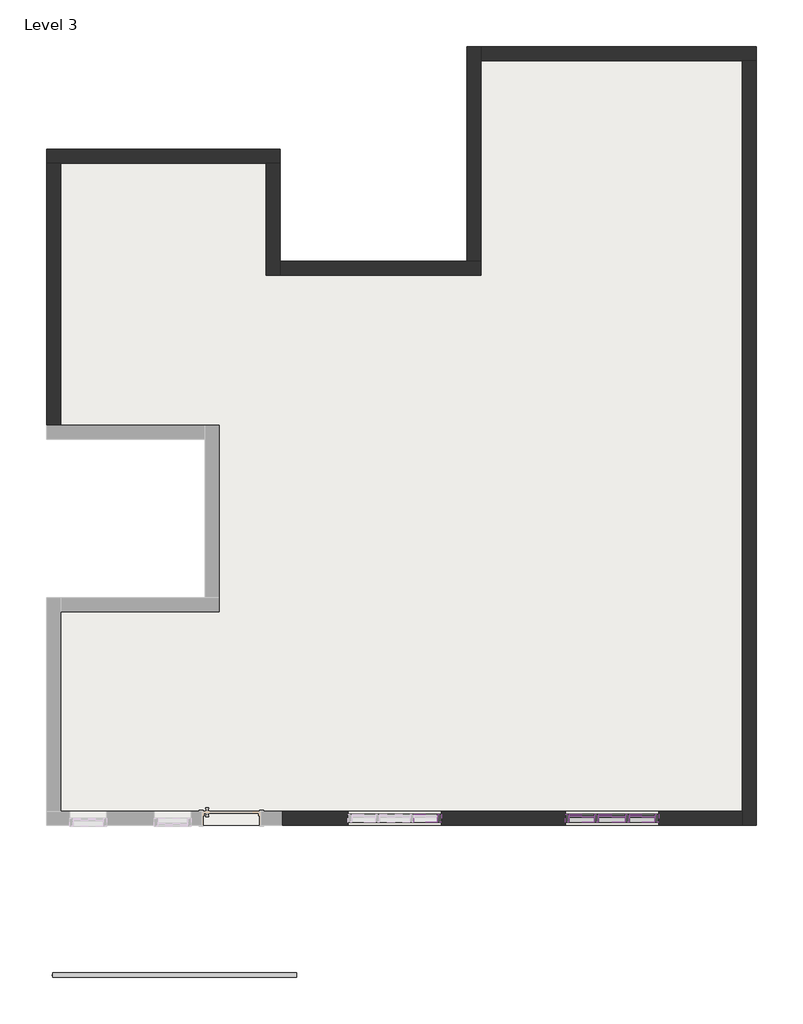
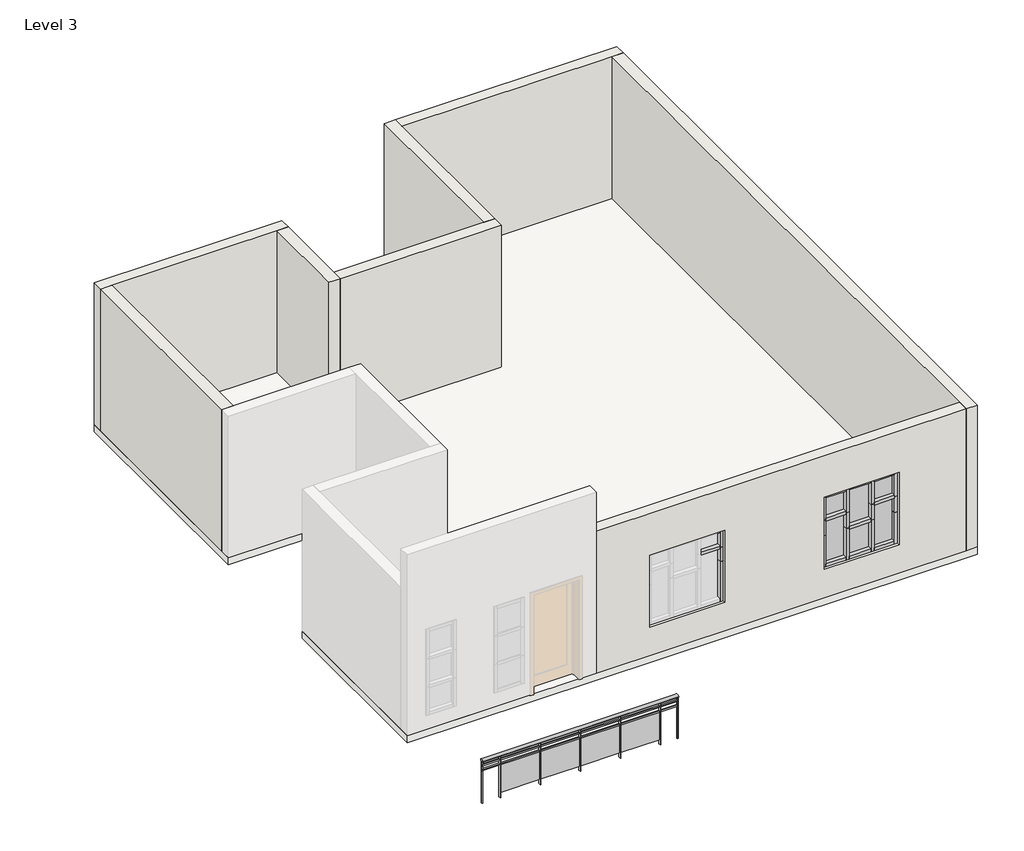
# One storey, part 2 of 2: 25 members, 8 walls, 6 plates, 1 railing, 1 slab.
"""IFC4 building model written with IfcOpenShell, lengths in millimetres."""

from ifc_helpers import new_model, si_unit, point, frame, origin, place, context, project, spatial, polyline, ellipse_curve, trimmed, outline, extrude, faceted_brep, transform, mapped, element, save
from ifc_brep_helpers import plane_surface, extruded_surface, advanced_brep
from components import member_3709dd30, member_b70ee1cc, member_3c3dc66a, member_dfe75557, member_dc106669, member_6428e230, member_5ae8a700, member_718fe5d9, member_bc7dbe04, member_b2812fca, member_26d576e8, member_fb4dac25, member_bdfbb35d, member_b281fab0, system_panel_glazed_1c8147a1, system_panel_glazed_d072c6ac, system_panel_glazed_ee3fb3da, system_panel_glazed_af2b4658

model = new_model("IFC4")

# Units and contexts
model_context = context("Model", 3, world=origin())
ifc_project = project(units=[si_unit("LENGTHUNIT", "METRE", prefix="MILLI")], contexts=[model_context])

# Site, building, storey
site = spatial("IfcSite", under=ifc_project)
building = spatial("IfcBuilding", under=site)
storey = spatial("IfcBuildingStorey", under=building, Name="Level 3", Elevation=3810.0)

# Members
placement = place(None, origin())
member_shape = member_3709dd30(model_context)
element("IfcMember", 1, ObjectType="Rectangular Mullion : 2.5\" x 5\" rectangular", at=placement, inside=storey, context=model_context, shape_type="MappedRepresentation", body=[
    mapped(member_shape, transform((-5777.6179297, 28.9196292, 5588.0), x_axis=(0.0, 0.0, 1.0), y_axis=(0.0, -1.0, 0.0), z_axis=(1.0, 0.0, 0.0))),
])
member_2_shape = member_b70ee1cc(model_context)
element("IfcMember", 2, ObjectType="Rectangular Mullion : 2.5\" x 5\" rectangular", at=placement, inside=storey, context=model_context, shape_type="MappedRepresentation", body=[
    mapped(member_2_shape, transform((-5714.1179297, 28.9196292, 4419.6), x_axis=(1.0, 0.0, 0.0), y_axis=(0.0, -1.0, 0.0), z_axis=(0.0, 0.0, -1.0))),
])
member_3_shape = member_3c3dc66a(model_context)
element("IfcMember", 3, ObjectType="Rectangular Mullion : 2.5\" x 5\" rectangular", at=placement, inside=storey, context=model_context, shape_type="MappedRepresentation", body=[
    mapped(member_3_shape, transform((-5714.1179297, 28.9196292, 5283.2), x_axis=(1.0, 0.0, 0.0), y_axis=(0.0, -1.0, 0.0), z_axis=(0.0, 0.0, -1.0))),
])
member_4_shape = member_dfe75557(model_context)
element("IfcMember", 4, ObjectType="Rectangular Mullion : 2.5\" x 5\" rectangular", at=placement, inside=storey, context=model_context, shape_type="MappedRepresentation", body=[
    mapped(member_4_shape, transform((-5714.1179297, 28.9196292, 5588.0), x_axis=(1.0, 0.0, 0.0), y_axis=(0.0, -1.0, 0.0), z_axis=(0.0, 0.0, -1.0))),
])
member_5_shape = member_dc106669(model_context)
element("IfcMember", 5, ObjectType="Rectangular Mullion : 2.5\" x 5\" rectangular", at=placement, inside=storey, context=model_context, shape_type="MappedRepresentation", body=[
    mapped(member_5_shape, transform((-2234.3179297, 28.9196292, 5969.0), x_axis=(0.0, 0.0, 1.0), y_axis=(0.0, -1.0, 0.0), z_axis=(1.0, 0.0, 0.0))),
])
element("IfcMember", 6, ObjectType="Rectangular Mullion : 2.5\" x 5\" rectangular", at=placement, inside=storey, context=model_context, shape_type="MappedRepresentation", body=[
    mapped(member_5_shape, transform((-3218.5679297, 28.9196292, 5969.0), x_axis=(0.0, 0.0, 1.0), y_axis=(0.0, -1.0, 0.0), z_axis=(1.0, 0.0, 0.0))),
])
element("IfcMember", 7, ObjectType="Rectangular Mullion : 2.5\" x 5\" rectangular", at=placement, inside=storey, context=model_context, shape_type="MappedRepresentation", body=[
    mapped(member_5_shape, transform((-3631.3179297, 28.9196292, 4419.6), x_axis=(0.0, 0.0, -1.0), y_axis=(0.0, -1.0, 0.0), z_axis=(-1.0, 0.0, 0.0))),
])
element("IfcMember", 8, ObjectType="Rectangular Mullion : 2.5\" x 5\" rectangular", at=placement, inside=storey, context=model_context, shape_type="MappedRepresentation", body=[
    mapped(member_5_shape, transform((-2647.0679297, 28.9196292, 4419.6), x_axis=(0.0, 0.0, -1.0), y_axis=(0.0, -1.0, 0.0), z_axis=(-1.0, 0.0, 0.0))),
])
member_6_shape = member_6428e230(model_context)
element("IfcMember", 9, ObjectType="Rectangular Mullion : 2.5\" x 5\" rectangular", at=placement, inside=storey, context=model_context, shape_type="MappedRepresentation", body=[
    mapped(member_6_shape, transform((-3186.8179297, 28.9196292, 4419.6), x_axis=(1.0, 0.0, 0.0), y_axis=(0.0, -1.0, 0.0), z_axis=(0.0, 0.0, -1.0))),
])
element("IfcMember", 10, ObjectType="Rectangular Mullion : 2.5\" x 5\" rectangular", at=placement, inside=storey, context=model_context, shape_type="MappedRepresentation", body=[
    mapped(member_6_shape, transform((-2678.8179297, 28.9196292, 4419.6), x_axis=(1.0, 0.0, 0.0), y_axis=(0.0, -1.0, 0.0), z_axis=(0.0, 0.0, -1.0))),
])
member_7_shape = member_5ae8a700(model_context)
element("IfcMember", 11, ObjectType="Rectangular Mullion : 2.5\" x 5\" rectangular", at=placement, inside=storey, context=model_context, shape_type="MappedRepresentation", body=[
    mapped(member_7_shape, transform((-3218.5679297, 28.9196292, 5435.6), x_axis=(0.0, 0.0, 1.0), y_axis=(0.0, -1.0, 0.0), z_axis=(1.0, 0.0, 0.0))),
])
element("IfcMember", 12, ObjectType="Rectangular Mullion : 2.5\" x 5\" rectangular", at=placement, inside=storey, context=model_context, shape_type="MappedRepresentation", body=[
    mapped(member_7_shape, transform((-2234.3179297, 28.9196292, 5435.6), x_axis=(0.0, 0.0, 1.0), y_axis=(0.0, -1.0, 0.0), z_axis=(1.0, 0.0, 0.0))),
])
member_8_shape = member_718fe5d9(model_context)
element("IfcMember", 13, ObjectType="Rectangular Mullion : 2.5\" x 5\" rectangular", at=placement, inside=storey, context=model_context, shape_type="MappedRepresentation", body=[
    mapped(member_8_shape, transform((-2710.5679297, 28.9196292, 5096.9333333), x_axis=(0.0, 0.0, 1.0), y_axis=(0.0, -1.0, 0.0), z_axis=(1.0, 0.0, 0.0))),
])
member_9_shape = member_bc7dbe04(model_context)
element("IfcMember", 14, ObjectType="Rectangular Mullion : 2.5\" x 5\" rectangular", at=placement, inside=storey, context=model_context, shape_type="MappedRepresentation", body=[
    mapped(member_9_shape, transform((-3155.0679297, 28.9196292, 4419.6), x_axis=(0.0, 0.0, -1.0), y_axis=(0.0, -1.0, 0.0), z_axis=(-1.0, 0.0, 0.0))),
])
element("IfcMember", 15, ObjectType="Rectangular Mullion : 2.5\" x 5\" rectangular", at=placement, inside=storey, context=model_context, shape_type="MappedRepresentation", body=[
    mapped(member_9_shape, transform((-2710.5679297, 28.9196292, 5969.0), x_axis=(0.0, 0.0, 1.0), y_axis=(0.0, -1.0, 0.0), z_axis=(1.0, 0.0, 0.0))),
])
member_10_shape = member_b2812fca(model_context)
element("IfcMember", 16, ObjectType="Rectangular Mullion : 2.5\" x 5\" rectangular", at=placement, inside=storey, context=model_context, shape_type="MappedRepresentation", body=[
    mapped(member_10_shape, transform((-3186.8179297, 28.9196292, 5096.9333333), x_axis=(1.0, 0.0, 0.0), y_axis=(0.0, -1.0, 0.0), z_axis=(0.0, 0.0, -1.0))),
])
element("IfcMember", 17, ObjectType="Rectangular Mullion : 2.5\" x 5\" rectangular", at=placement, inside=storey, context=model_context, shape_type="MappedRepresentation", body=[
    mapped(member_10_shape, transform((-2678.8179297, 28.9196292, 5096.9333333), x_axis=(1.0, 0.0, 0.0), y_axis=(0.0, -1.0, 0.0), z_axis=(0.0, 0.0, -1.0))),
])
member_11_shape = member_26d576e8(model_context)
element("IfcMember", 18, ObjectType="Rectangular Mullion : 2.5\" x 5\" rectangular", at=placement, inside=storey, context=model_context, shape_type="MappedRepresentation", body=[
    mapped(member_11_shape, transform((-2170.8179297, 28.9196292, 4419.6), x_axis=(1.0, 0.0, 0.0), y_axis=(0.0, -1.0, 0.0), z_axis=(0.0, 0.0, -1.0))),
])
member_12_shape = member_fb4dac25(model_context)
element("IfcMember", 19, ObjectType="Rectangular Mullion : 2.5\" x 5\" rectangular", at=placement, inside=storey, context=model_context, shape_type="MappedRepresentation", body=[
    mapped(member_12_shape, transform((-2170.8179297, 28.9196292, 5096.9333333), x_axis=(1.0, 0.0, 0.0), y_axis=(0.0, -1.0, 0.0), z_axis=(0.0, 0.0, -1.0))),
])
element("IfcMember", 20, ObjectType="Rectangular Mullion : 2.5\" x 5\" rectangular", at=placement, inside=storey, context=model_context, shape_type="MappedRepresentation", body=[
    mapped(member_12_shape, transform((-3694.8179297, 28.9196292, 5435.6), x_axis=(-1.0, 0.0, 0.0), y_axis=(0.0, -1.0, 0.0), z_axis=(0.0, 0.0, 1.0))),
])
element("IfcMember", 21, ObjectType="Rectangular Mullion : 2.5\" x 5\" rectangular", at=placement, inside=storey, context=model_context, shape_type="MappedRepresentation", body=[
    mapped(member_11_shape, transform((-3694.8179297, 28.9196292, 5096.9333333), x_axis=(-1.0, 0.0, 0.0), y_axis=(0.0, -1.0, 0.0), z_axis=(0.0, 0.0, 1.0))),
])
member_13_shape = member_bdfbb35d(model_context)
element("IfcMember", 22, ObjectType="Rectangular Mullion : 2.5\" x 5\" rectangular", at=placement, inside=storey, context=model_context, shape_type="MappedRepresentation", body=[
    mapped(member_13_shape, transform((-3186.8179297, 28.9196292, 5435.6), x_axis=(1.0, 0.0, 0.0), y_axis=(0.0, -1.0, 0.0), z_axis=(0.0, 0.0, -1.0))),
])
element("IfcMember", 23, ObjectType="Rectangular Mullion : 2.5\" x 5\" rectangular", at=placement, inside=storey, context=model_context, shape_type="MappedRepresentation", body=[
    mapped(member_13_shape, transform((-2678.8179297, 28.9196292, 5435.6), x_axis=(1.0, 0.0, 0.0), y_axis=(0.0, -1.0, 0.0), z_axis=(0.0, 0.0, -1.0))),
])
member_14_shape = member_b281fab0(model_context)
element("IfcMember", 24, ObjectType="Rectangular Mullion : 2.5\" x 5\" rectangular", at=placement, inside=storey, context=model_context, shape_type="MappedRepresentation", body=[
    mapped(member_14_shape, transform((-3694.8179297, 28.9196292, 5969.0), x_axis=(-1.0, 0.0, 0.0), y_axis=(0.0, -1.0, 0.0), z_axis=(0.0, 0.0, 1.0))),
])
element("IfcMember", 25, ObjectType="Rectangular Mullion : 2.5\" x 5\" rectangular", at=placement, inside=storey, context=model_context, shape_type="MappedRepresentation", body=[
    mapped(member_14_shape, transform((-2170.8179297, 28.9196292, 5435.6), x_axis=(1.0, 0.0, 0.0), y_axis=(0.0, -1.0, 0.0), z_axis=(0.0, 0.0, -1.0))),
])

# Plates
system_panel_glazed_shape = system_panel_glazed_1c8147a1(model_context)
element("IfcPlate", 26, ObjectType="System Panel : Glazed", at=placement, inside=storey, context=model_context, shape_type="MappedRepresentation", body=[
    mapped(system_panel_glazed_shape, transform((-3424.9429297, 28.9196292, 4483.1), x_axis=(1.0, 0.0, 0.0), y_axis=(0.0, 1.0, 0.0), z_axis=(0.0, 0.0, 1.0))),
])
element("IfcPlate", 27, ObjectType="System Panel : Glazed", at=placement, inside=storey, context=model_context, shape_type="MappedRepresentation", body=[
    mapped(system_panel_glazed_shape, transform((-2440.6929297, 28.9196292, 4483.1), x_axis=(1.0, 0.0, 0.0), y_axis=(0.0, 1.0, 0.0), z_axis=(0.0, 0.0, 1.0))),
])
system_panel_glazed_2_shape = system_panel_glazed_d072c6ac(model_context)
element("IfcPlate", 28, ObjectType="System Panel : Glazed", at=placement, inside=storey, context=model_context, shape_type="MappedRepresentation", body=[
    mapped(system_panel_glazed_2_shape, transform((-2932.8179297, 28.9196292, 4483.1), x_axis=(1.0, 0.0, 0.0), y_axis=(0.0, 1.0, 0.0), z_axis=(0.0, 0.0, 1.0))),
])
system_panel_glazed_3_shape = system_panel_glazed_ee3fb3da(model_context)
element("IfcPlate", 29, ObjectType="System Panel : Glazed", at=placement, inside=storey, context=model_context, shape_type="MappedRepresentation", body=[
    mapped(system_panel_glazed_3_shape, transform((-3424.9429297, 28.9196292, 5467.35), x_axis=(1.0, 0.0, 0.0), y_axis=(0.0, 1.0, 0.0), z_axis=(0.0, 0.0, 1.0))),
])
element("IfcPlate", 30, ObjectType="System Panel : Glazed", at=placement, inside=storey, context=model_context, shape_type="MappedRepresentation", body=[
    mapped(system_panel_glazed_3_shape, transform((-2440.6929297, 28.9196292, 5467.35), x_axis=(1.0, 0.0, 0.0), y_axis=(0.0, 1.0, 0.0), z_axis=(0.0, 0.0, 1.0))),
])
system_panel_glazed_4_shape = system_panel_glazed_af2b4658(model_context)
element("IfcPlate", 31, ObjectType="System Panel : Glazed", at=placement, inside=storey, context=model_context, shape_type="MappedRepresentation", body=[
    mapped(system_panel_glazed_4_shape, transform((-2932.8179297, 28.9196292, 5128.6833333), x_axis=(1.0, 0.0, 0.0), y_axis=(0.0, 1.0, 0.0), z_axis=(0.0, 0.0, 1.0))),
])

# Railing
element("IfcRailing", 32, ObjectType="Glass Panel - Bottom Fill", at=placement, inside=storey, context=model_context, shape_type="SolidModel", body=[
    advanced_brep(
    [(-8082.6679297, -2567.1989686, 4724.4), (-8082.6679297, -2490.9989686, 4724.4), (-12057.7679297, -2567.1989686, 4724.4), (-12057.7679297, -2490.9989686, 4724.4)],
    [
        (0, 1, ellipse_curve(frame((-8082.6679297, -2529.0989686, 4724.4), z_axis=(1.0, 0.0, 0.0), x_axis=(0.0, 1.0, 0.0)), 38.1, 28.575)),
        (1, 0, ellipse_curve(frame((-8082.6679297, -2529.0989686, 4724.4), z_axis=(1.0, 0.0, 0.0), x_axis=(0.0, 1.0, 0.0)), 38.1, 28.575)),
        (2, 3, ellipse_curve(frame((-12057.7679297, -2529.0989686, 4724.4), z_axis=(-1.0, 0.0, 0.0), x_axis=(0.0, 1.0, 0.0)), 38.1, 28.575)),
        (3, 2, ellipse_curve(frame((-12057.7679297, -2529.0989686, 4724.4), z_axis=(-1.0, 0.0, 0.0), x_axis=(0.0, 1.0, 0.0)), 38.1, 28.575)),
        (0, 2),
        (3, 1),
    ],
    [
        plane_surface(frame((-8082.6679297, -2529.0989686, 4724.4), z_axis=(1.0, 0.0, 0.0), x_axis=(0.0, -1.0, 0.0))),
        plane_surface(frame((-12057.7679297, -2529.0989686, 4724.4), z_axis=(-1.0, 0.0, 0.0), x_axis=(0.0, -1.0, 0.0))),
        extruded_surface(trimmed(ellipse_curve(frame((-12057.7679297, -2529.0989686, 4724.4), z_axis=(1.0, 0.0, 0.0), x_axis=(0.0, 1.0, 0.0)), 38.1, 28.575), [point((-12057.7679297, -2567.1989686, 4724.4))], [point((-12057.7679297, -2490.9989686, 4724.4))], True, "CARTESIAN"), (3975.0999999999995, 0.0, 0.0), 3975.0999999999995),
        extruded_surface(trimmed(ellipse_curve(frame((-12057.7679297, -2529.0989686, 4724.4), z_axis=(1.0, 0.0, 0.0), x_axis=(0.0, 1.0, 0.0)), 38.1, 28.575), [point((-12057.7679297, -2490.9989686, 4724.4))], [point((-12057.7679297, -2567.1989686, 4724.4))], True, "CARTESIAN"), (3975.0999999999995, 0.0, 0.0), 3975.0999999999995),
    ],
    [
        (0, [[1, 2]]),
        (1, [[3, 4]]),
        (2, [[-1, 5, -4, 6]]),
        (3, [[-2, -6, -3, -5]]),
    ],
),
    extrude(outline(polyline([(-8082.6679297, -2516.3989686), (-8082.6679297, -2541.7989686), (-12057.7679297, -2541.7989686), (-12057.7679297, -2516.3989686), (-8082.6679297, -2516.3989686)])), frame((0.0, 0.0, 4610.1), z_axis=(0.0, 0.0, 1.0), x_axis=(1.0, 0.0, 0.0)), (0.0, 0.0, 1.0), 25.4),
    extrude(outline(polyline([(-8082.6679297, -2516.3989686), (-8082.6679297, -2541.7989686), (-12057.7679297, -2541.7989686), (-12057.7679297, -2516.3989686), (-8082.6679297, -2516.3989686)])), frame((0.0, 0.0, 4508.5), z_axis=(0.0, 0.0, 1.0), x_axis=(1.0, 0.0, 0.0)), (0.0, 0.0, 1.0), 25.4),
    extrude(outline(polyline([(-11689.4679297, -2503.6989686), (-11689.4679297, -2554.4989686), (-11702.1679297, -2554.4989686), (-11702.1679297, -2503.6989686), (-11689.4679297, -2503.6989686)])), frame((0.0, 0.0, 3810.0), z_axis=(0.0, 0.0, 1.0), x_axis=(1.0, 0.0, 0.0)), (0.0, 0.0, 1.0), 885.825),
    extrude(outline(polyline([(-10883.0179297, -2535.6341256), (-11695.8179297, -2535.6341256), (-11695.8179297, -2529.2841256), (-10883.0179297, -2529.2841256), (-10883.0179297, -2535.6341256)])), frame((0.0, 0.0, 3911.6), z_axis=(0.0, 0.0, 1.0), x_axis=(1.0, 0.0, 0.0)), (0.0, 0.0, 1.0), 596.9),
    extrude(outline(polyline([(-10876.6679297, -2503.6989686), (-10876.6679297, -2554.4989686), (-10889.3679297, -2554.4989686), (-10889.3679297, -2503.6989686), (-10876.6679297, -2503.6989686)])), frame((0.0, 0.0, 3810.0), z_axis=(0.0, 0.0, 1.0), x_axis=(1.0, 0.0, 0.0)), (0.0, 0.0, 1.0), 885.825),
    extrude(outline(polyline([(-10070.2179297, -2535.6341256), (-10883.0179297, -2535.6341256), (-10883.0179297, -2529.2841256), (-10070.2179297, -2529.2841256), (-10070.2179297, -2535.6341256)])), frame((0.0, 0.0, 3911.6), z_axis=(0.0, 0.0, 1.0), x_axis=(1.0, 0.0, 0.0)), (0.0, 0.0, 1.0), 596.9),
    extrude(outline(polyline([(-10063.8679297, -2503.6989686), (-10063.8679297, -2554.4989686), (-10076.5679297, -2554.4989686), (-10076.5679297, -2503.6989686), (-10063.8679297, -2503.6989686)])), frame((0.0, 0.0, 3810.0), z_axis=(0.0, 0.0, 1.0), x_axis=(1.0, 0.0, 0.0)), (0.0, 0.0, 1.0), 885.825),
    extrude(outline(polyline([(-9257.4179297, -2535.6341256), (-10070.2179297, -2535.6341256), (-10070.2179297, -2529.2841256), (-9257.4179297, -2529.2841256), (-9257.4179297, -2535.6341256)])), frame((0.0, 0.0, 3911.6), z_axis=(0.0, 0.0, 1.0), x_axis=(1.0, 0.0, 0.0)), (0.0, 0.0, 1.0), 596.9),
    extrude(outline(polyline([(-9251.0679297, -2503.6989686), (-9251.0679297, -2554.4989686), (-9263.7679297, -2554.4989686), (-9263.7679297, -2503.6989686), (-9251.0679297, -2503.6989686)])), frame((0.0, 0.0, 3810.0), z_axis=(0.0, 0.0, 1.0), x_axis=(1.0, 0.0, 0.0)), (0.0, 0.0, 1.0), 885.825),
    extrude(outline(polyline([(-8444.6179297, -2535.6341256), (-9257.4179297, -2535.6341256), (-9257.4179297, -2529.2841256), (-8444.6179297, -2529.2841256), (-8444.6179297, -2535.6341256)])), frame((0.0, 0.0, 3911.6), z_axis=(0.0, 0.0, 1.0), x_axis=(1.0, 0.0, 0.0)), (0.0, 0.0, 1.0), 596.9),
    extrude(outline(polyline([(-8438.2679297, -2503.6989686), (-8438.2679297, -2554.4989686), (-8450.9679297, -2554.4989686), (-8450.9679297, -2503.6989686), (-8438.2679297, -2503.6989686)])), frame((0.0, 0.0, 3810.0), z_axis=(0.0, 0.0, 1.0), x_axis=(1.0, 0.0, 0.0)), (0.0, 0.0, 1.0), 885.825),
    extrude(outline(polyline([(-12045.0679297, -2519.5739686), (-12045.0679297, -2538.6239686), (-12064.1179297, -2538.6239686), (-12064.1179297, -2519.5739686), (-12045.0679297, -2519.5739686)])), frame((0.0, 0.0, 3810.0), z_axis=(0.0, 0.0, 1.0), x_axis=(1.0, 0.0, 0.0)), (0.0, 0.0, 1.0), 885.825),
    extrude(outline(polyline([(-8076.3179297, -2519.5739686), (-8076.3179297, -2538.6239686), (-8095.3679297, -2538.6239686), (-8095.3679297, -2519.5739686), (-8076.3179297, -2519.5739686)])), frame((0.0, 0.0, 3810.0), z_axis=(0.0, 0.0, 1.0), x_axis=(1.0, 0.0, 0.0)), (0.0, 0.0, 1.0), 885.825),
])

# Slab
element("IfcSlab", 33, ObjectType="6\" floor", at=placement, inside=storey, context=model_context, shape_type="SweptSolid", body=[
    extrude(outline(polyline([(-12159.3679297, 10938.2196292), (-8349.3679297, 10938.2196292), (-8349.3679297, 9109.4196292), (-5301.3679297, 9109.4196292), (-5301.3679297, 12614.6196292), (-576.9679297, 12614.6196292), (-576.9679297, -85.3803708), (-12159.3679297, -85.3803708), (-12159.3679297, 3623.0196292), (-9568.5679297, 3623.0196292), (-9568.5679297, 6213.8196292), (-12159.3679297, 6213.8196292), (-12159.3679297, 10938.2196292)])), frame((0.0, 0.0, 3657.6), z_axis=(0.0, 0.0, 1.0), x_axis=(1.0, 0.0, 0.0)), (0.0, 0.0, 1.0), 152.4),
])

# Walls
element("IfcWall", 34, ObjectType="9\" wall", at=placement, inside=storey, context=model_context, shape_type="Brep", body=[
    faceted_brep([(-12159.3679297, 10709.6196292, 3810.0), (-11930.7679297, 10709.6196292, 3810.0), (-8577.9679297, 10709.6196292, 3810.0), (-8349.3679297, 10709.6196292, 3810.0), (-8349.3679297, 10709.6196292, 6858.0), (-8577.9679297, 10709.6196292, 6858.0), (-11930.7679297, 10709.6196292, 6858.0), (-12159.3679297, 10709.6196292, 6858.0), (-12159.3679297, 10938.2196292, 3810.0), (-12159.3679297, 10938.2196292, 6858.0), (-8349.3679297, 10938.2196292, 6858.0), (-8349.3679297, 10938.2196292, 3810.0)], [[[0, 1, 2, 3, 4, 5, 6, 7]], [[8, 9, 10, 11]], [[3, 2, 1, 0, 8, 11]], [[7, 6, 5, 4, 10, 9]], [[4, 3, 11, 10]], [[0, 7, 9, 8]]]),
])
element("IfcWall", 35, ObjectType="9\" wall", at=placement, inside=storey, context=model_context, shape_type="Brep", body=[
    faceted_brep([(-8577.9679297, 10709.6196292, 3810.0), (-8577.9679297, 8880.8196292, 3810.0), (-8577.9679297, 8880.8196292, 6858.0), (-8577.9679297, 10709.6196292, 6858.0), (-8349.3679297, 10709.6196292, 3810.0), (-8349.3679297, 10709.6196292, 6858.0), (-8349.3679297, 9109.4196292, 6858.0), (-8349.3679297, 8880.8196292, 6858.0), (-8349.3679297, 8880.8196292, 3810.0), (-8349.3679297, 9109.4196292, 3810.0)], [[[0, 1, 2, 3]], [[4, 5, 6, 7, 8, 9]], [[1, 0, 4, 9, 8]], [[3, 2, 7, 6, 5]], [[0, 3, 5, 4]], [[2, 1, 8, 7]]]),
])
element("IfcWall", 36, ObjectType="9\" wall", at=placement, inside=storey, context=model_context, shape_type="Brep", body=[
    faceted_brep([(-8349.3679297, 8880.8196292, 3810.0), (-5072.7679297, 8880.8196292, 3810.0), (-5072.7679297, 8880.8196292, 6858.0), (-8349.3679297, 8880.8196292, 6858.0), (-8349.3679297, 9109.4196292, 3810.0), (-8349.3679297, 9109.4196292, 6858.0), (-5301.3679297, 9109.4196292, 6858.0), (-5072.7679297, 9109.4196292, 6858.0), (-5072.7679297, 9109.4196292, 3810.0), (-5301.3679297, 9109.4196292, 3810.0)], [[[0, 1, 2, 3]], [[4, 5, 6, 7, 8, 9]], [[1, 0, 4, 9, 8]], [[3, 2, 7, 6, 5]], [[0, 3, 5, 4]], [[2, 1, 8, 7]]]),
])
element("IfcWall", 37, ObjectType="9\" wall", at=placement, inside=storey, context=model_context, shape_type="Brep", body=[
    faceted_brep([(-5072.7679297, 9109.4196292, 3810.0), (-5072.7679297, 12386.0196292, 3810.0), (-5072.7679297, 12614.6196292, 3810.0), (-5072.7679297, 12614.6196292, 6858.0), (-5072.7679297, 12386.0196292, 6858.0), (-5072.7679297, 9109.4196292, 6858.0), (-5301.3679297, 9109.4196292, 3810.0), (-5301.3679297, 9109.4196292, 6858.0), (-5301.3679297, 12614.6196292, 6858.0), (-5301.3679297, 12614.6196292, 3810.0)], [[[0, 1, 2, 3, 4, 5]], [[6, 7, 8, 9]], [[2, 1, 0, 6, 9]], [[5, 4, 3, 8, 7]], [[0, 5, 7, 6]], [[3, 2, 9, 8]]]),
])
element("IfcWall", 38, ObjectType="9\" wall", at=placement, inside=storey, context=model_context, shape_type="Brep", body=[
    faceted_brep([(-5072.7679297, 12386.0196292, 3810.0), (-805.5679297, 12386.0196292, 3810.0), (-576.9679297, 12386.0196292, 3810.0), (-576.9679297, 12386.0196292, 6858.0), (-805.5679297, 12386.0196292, 6858.0), (-5072.7679297, 12386.0196292, 6858.0), (-5072.7679297, 12614.6196292, 3810.0), (-5072.7679297, 12614.6196292, 6858.0), (-576.9679297, 12614.6196292, 6858.0), (-576.9679297, 12614.6196292, 3810.0)], [[[0, 1, 2, 3, 4, 5]], [[6, 7, 8, 9]], [[2, 1, 0, 6, 9]], [[5, 4, 3, 8, 7]], [[0, 5, 7, 6]], [[3, 2, 9, 8]]]),
])
element("IfcWall", 39, ObjectType="9\" wall", at=placement, inside=storey, context=model_context, shape_type="Brep", body=[
    faceted_brep([(-805.5679297, 12386.0196292, 3810.0), (-805.5679297, 143.2196292, 3810.0), (-805.5679297, -85.3803708, 3810.0), (-805.5679297, -85.3803708, 6858.0), (-805.5679297, 143.2196292, 6858.0), (-805.5679297, 12386.0196292, 6858.0), (-576.9679297, 12386.0196292, 3810.0), (-576.9679297, 12386.0196292, 6858.0), (-576.9679297, -85.3803708, 6858.0), (-576.9679297, -85.3803708, 3810.0)], [[[0, 1, 2, 3, 4, 5]], [[6, 7, 8, 9]], [[2, 1, 0, 6, 9]], [[5, 4, 3, 8, 7]], [[0, 5, 7, 6]], [[3, 2, 9, 8]]]),
])
element("IfcWall", 40, ObjectType="9\" wall", at=placement, inside=storey, context=model_context, shape_type="SweptSolid", body=[
    extrude(outline(polyline([(3810.0, -8317.6179297), (3810.0, -805.5679297), (6858.0, -805.5679297), (6858.0, -8317.6179297), (3810.0, -8317.6179297)]), holes=[polyline([(4419.6, -7238.1179297), (5969.0, -7238.1179297), (5969.0, -5714.1179297), (4419.6, -5714.1179297), (4419.6, -7238.1179297)]), polyline([(4419.6, -3694.8179297), (5969.0, -3694.8179297), (5969.0, -2170.8179297), (4419.6, -2170.8179297), (4419.6, -3694.8179297)])]), frame((0.0, -85.3803708, 0.0), z_axis=(0.0, 1.0, 0.0), x_axis=(0.0, 0.0, 1.0)), (0.0, 0.0, 1.0), 228.6),
])
element("IfcWall", 41, ObjectType="9\" wall", at=placement, inside=storey, context=model_context, shape_type="SweptSolid", body=[
    extrude(outline(polyline([(-11930.7679297, 10709.6196292), (-11930.7679297, 6442.4196292), (-12159.3679297, 6442.4196292), (-12159.3679297, 10709.6196292), (-11930.7679297, 10709.6196292)])), frame((0.0, 0.0, 3810.0), z_axis=(0.0, 0.0, 1.0), x_axis=(1.0, 0.0, 0.0)), (0.0, 0.0, 1.0), 3048.0),
])

save(model, "model.ifc")

# Revit data of these elements
# Type "Rectangular Mullion : 2.5\" x 5\" rectangular"
#   built-in parameter 1007304 = 0.416667 (stored number, unit not read)
#   built-in parameter 1007301 = 0.104167 (stored number, unit not read)
#   built-in parameter 1007300 = 0.104167 (stored number, unit not read)
# Type "System Panel : Glazed"
#   Construction Type Id = "GSP4R"
#   Analytic Construction = "1/8 in Pilkington single glazing"
#   Visual Light Transmittance = 0.9
#   Solar Heat Gain Coefficient = 0.86
#   Heat Transfer Coefficient (U) = 1.18115 BTU/(h·ft²·°F)
#   Define Thermal Properties by = 1
# Type "Glass Panel - Bottom Fill"
#   Assembly Code = "C2010400"
#   built-in parameter 1008612 = 0.0416667 (stored number, unit not read)
#   built-in parameter 1008611 = 0.0416667 (stored number, unit not read)
#   built-in parameter 1008609 = 0.333333 (stored number, unit not read)
#   built-in parameter 1008604 = 0.166667 (stored number, unit not read)
#   built-in parameter 1008603 = 0.166667 (stored number, unit not read)
#   Railing Height = 3' - 0"
#   built-in parameter 1008630 = 2
#   built-in parameter 1008610 = 2
#   built-in parameter 1008618 = Baluster - Square : 3/4"
# Type "6\" floor"
#   Assembly Code = "B1010"
#   Function = 0
#   Layers, outside or top first: 0' - 6" "Laminate, Ivory, Matte" (function 1)
# Type "9\" wall"
#   Assembly Code = "B2010"
#   Layers, outside or top first: 0' - 9" "Laminate, Ivory, Matte" (function 1)
# Elements 1, 2, 3, 4, 5, 6, 7, 8, 9, 10, 11, 12, 13, 14, 15, 16, 17, 18, 19, 20, 21, 22, 23, 24, 25 (IfcMember, "Rectangular Mullion : 2.5\" x 5\" rectangular")
#   Phase Created = New Construction
#   Materials on its faces: "door colour"
# Elements 26, 27, 28, 29, 30, 31 (IfcPlate, "System Panel : Glazed")
#   Phase Created = New Construction
#   Materials on its faces: "Glass"
# Element 32 (IfcRailing, "Glass Panel - Bottom Fill")
#   Phase Created = New Construction
#   Materials on its faces: "Glass", "Iron, Ductile"
# Element 33 (IfcSlab, "6\" floor")
#   built-in parameter 1001955 = 3.14159 (stored number, unit not read)
#   Height Offset From Level = 0' - 0"
#   Phase Created = New Construction
#   Materials on its faces: "Laminate, Ivory, Matte"
# Elements 34, 35, 36, 37, 38, 39, 40, 41 (IfcWall, "9\" wall")
#   Top Offset = 0' - 0"
#   Base Offset = 0' - 0"
#   wall height = 10' - 0"
#   Phase Created = New Construction
#   Base Constraint = Level 3
#   Top Constraint = Level 4
#   Materials on its faces: "Laminate, Ivory, Matte"
# Materials
#   "Laminate, Ivory, Matte": class "Plastic", colour RGB 247 247 239, transparency 0, Description = "Plastic Laminate - Ivory, Matte", Cost = 0
#   "door colour": class "Generic", colour RGB 120 120 120, transparency 0, Cost = 0
#   "Glass": class "Glass", colour RGB 0 128 192, transparency 0.75, Description = "Soda Lime Glass", Cost = 0
#   "Iron, Ductile": class "Metal", colour RGB 0 0 0, transparency 0, Description = "Ductile cast iron", Cost = 0
